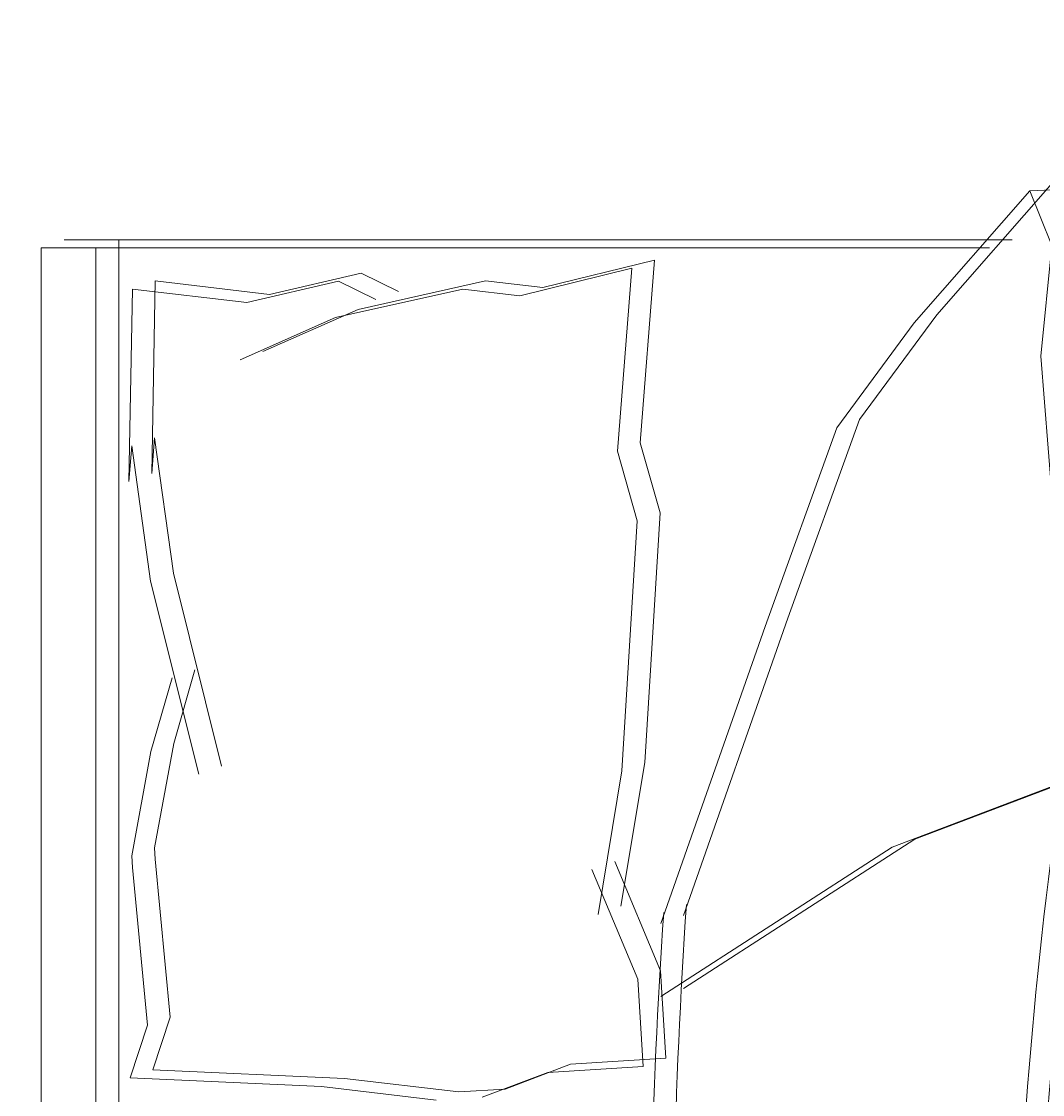
# Model space of a CAD drawing. Units: inches. Extents: x 1962 to 2771, y 1245 to 2660.
# Tile 45 of 114: x 2093 to 2116, y 2098 to 2122. Entities that reach past the tile are written whole.
import ezdxf

# ---------------------------------------------------------------- set-up
doc = ezdxf.new("R2010")
doc.units = ezdxf.units.IN
doc.layers.add('A-ANNO-DIMS', color=2, linetype='Continuous', lineweight=18)
doc.layers.add('A-FURN', color=8, linetype='Continuous', lineweight=13)
doc.styles.get("Standard").update_dxf_attribs({"font": 'arial.ttf'})
doc.dimstyles.get("Standard").update_dxf_attribs({"dimtxt": 0.18, "dimasz": 0.18, "dimexe": 0.18, "dimexo": 0.0625, "dimgap": 0.09, "dimtad": 0, "dimtih": 1, "dimtoh": 1, "dimdec": 4, "dimzin": 0, "dimdsep": 46, "dimtxsty": 'Standard', "dimcen": 0.09, "dimadec": 0, "dimazin": 0, "dimtfac": 1, "dimtdec": 4, "dimtofl": 0, "dimtmove": 0, "dimatfit": 3, "dimfxl": 1, "dimtolj": 1, "dimtzin": 0, "dimarcsym": 0})

# ---------------------------------------------------------------- blocks, each defined once
blk = doc.blocks.new('BED-PLAN')
for p, q in [((22.563, 42.207), (19.979, 39.261)), ((22.563, 42.206), (19.979, 39.261)), ((22.055, 42.025), (19.471, 39.08)), ((22.055, 42.025), (19.471, 39.08)), ((23.442, 42.088), (22.055, 42.025, 3.077)), ((23.442, 42.088), (22.055, 42.025, 3.077)), ((22.547, 40.803), (22.055, 42.025)), ((22.547, 40.803), (22.055, 42.025)), ((0.508, 40.933), (21.66, 40.933)), ((0.508, 40.933), (21.66, 40.933)), ((1.727, 2.945), (1.727, 40.933)), ((1.727, 2.945), (1.727, 40.933)), ((0, 40.752), (21.152, 40.752)), ((0, 40.751), (21.152, 40.751)), ((0, 2.764), (0, 40.751)), ((1.219, 2.764), (1.219, 40.752)), ((1.219, 2.763), (1.219, 40.751)), ((22.301, 38.341), (22.547, 40.803)), ((22.301, 38.341), (22.547, 40.803)), ((13.682, 40.482), (11.187, 39.866)), ((13.682, 40.482), (11.187, 39.866)), ((13.361, 36.403), (13.682, 40.482)), ((13.361, 36.403), (13.682, 40.482)), ((13.173, 40.301), (10.679, 39.684)), ((13.173, 40.301), (10.679, 39.684)), ((12.853, 36.222), (13.173, 40.301)), ((12.853, 36.221), (13.173, 40.301)), ((2.541, 40.016), (2.464, 35.722)), ((2.541, 40.016), (2.464, 35.722)), ((2.541, 40.016), (5.093, 39.715)), ((2.541, 40.016), (5.093, 39.715)), ((4.585, 39.534), (6.628, 40.007)), ((4.585, 39.533), (6.628, 40.007)), ((5.093, 39.715), (7.136, 40.188)), ((5.093, 39.715), (7.136, 40.188)), ((6.628, 40.007), (7.46, 39.598)), ((6.628, 40.007), (7.46, 39.598)), ((9.911, 40.016), (7.072, 39.378)), ((9.911, 40.016), (7.072, 39.378)), ((7.136, 40.188), (7.968, 39.78)), ((7.136, 40.188), (7.968, 39.78)), ((11.187, 39.866), (9.911, 40.016)), ((11.187, 39.866), (9.911, 40.016)), ((2.033, 39.835), (1.955, 35.54)), ((2.033, 39.834), (1.956, 35.54)), ((2.033, 39.835), (4.585, 39.534)), ((2.033, 39.834), (4.585, 39.533)), ((9.402, 39.835), (6.563, 39.197)), ((9.402, 39.835), (6.563, 39.197)), ((10.679, 39.684), (9.402, 39.835)), ((10.679, 39.684), (9.402, 39.835)), ((7.072, 39.378), (4.942, 38.439)), ((7.072, 39.378), (4.942, 38.439)), ((19.979, 39.261), (18.257, 36.922)), ((19.979, 39.261), (18.257, 36.922)), ((6.563, 39.197), (4.434, 38.258)), ((6.563, 39.197), (4.434, 38.258)), ((19.471, 39.08), (17.749, 36.741)), ((19.471, 39.08), (17.749, 36.741)), ((22.547, 35.263), (22.301, 38.341)), ((22.547, 35.263), (22.301, 38.341)), ((18.257, 36.922), (16.658, 32.49)), ((18.257, 36.922), (16.658, 32.49)), ((17.749, 36.741), (16.149, 32.309)), ((17.749, 36.741), (16.149, 32.309)), ((2.464, 35.722), (2.529, 36.519)), ((2.464, 35.722), (2.529, 36.519)), ((2.529, 36.519), (2.948, 33.5)), ((2.529, 36.519), (2.948, 33.5)), ((13.804, 34.845), (13.361, 36.403)), ((13.804, 34.845), (13.361, 36.403)), ((1.955, 35.54), (2.021, 36.338)), ((1.956, 35.54), (2.021, 36.337)), ((2.021, 36.338), (2.44, 33.319)), ((2.021, 36.337), (2.44, 33.318)), ((13.296, 34.663), (12.853, 36.222)), ((13.296, 34.663), (12.853, 36.221)), ((13.461, 29.273), (13.804, 34.845)), ((13.461, 29.273), (13.804, 34.845)), ((12.953, 29.091), (13.296, 34.663)), ((12.953, 29.091), (13.296, 34.663)), ((2.44, 33.319), (3.515, 29.011)), ((2.44, 33.318), (3.515, 29.011)), ((2.948, 33.5), (4.023, 29.192)), ((2.948, 33.5), (4.023, 29.192)), ((16.658, 32.49), (14.326, 25.863)), ((16.658, 32.49), (14.326, 25.862)), ((16.149, 32.309), (13.818, 25.681)), ((16.149, 32.309), (13.818, 25.681)), ((2.92, 31.161), (2.447, 29.52)), ((2.92, 31.161), (2.447, 29.519)), ((3.428, 31.343), (2.955, 29.701)), ((3.428, 31.342), (2.955, 29.701)), ((2.955, 29.701), (2.525, 27.372)), ((2.955, 29.701), (2.525, 27.372)), ((2.447, 29.52), (2.017, 27.19)), ((2.447, 29.519), (2.017, 27.19)), ((12.931, 26.068), (13.461, 29.273)), ((12.931, 26.068), (13.461, 29.273)), ((12.423, 25.886), (12.953, 29.091)), ((12.423, 25.886), (12.953, 29.091)), ((18.979, 27.385), (22.547, 28.739)), ((18.979, 27.384), (22.547, 28.739)), ((19.487, 27.566), (23.055, 28.92)), ((19.487, 27.566), (23.055, 28.92)), ((14.326, 24.236), (19.487, 27.566)), ((14.326, 24.235), (19.487, 27.566)), ((2.525, 27.372), (2.541, 27.117)), ((2.525, 27.372), (2.541, 27.116)), ((13.818, 24.054), (18.979, 27.385)), ((13.818, 24.054), (18.979, 27.384)), ((2.017, 27.19), (2.033, 26.935)), ((2.017, 27.19), (2.033, 26.935)), ((2.541, 27.117), (2.876, 23.597)), ((2.541, 27.116), (2.876, 23.597)), ((13.814, 24.626), (12.793, 27.067)), ((13.814, 24.626), (12.793, 27.066)), ((2.033, 26.935), (2.368, 23.415)), ((2.033, 26.935), (2.368, 23.415)), ((13.306, 24.444), (12.285, 26.885)), ((13.306, 24.444), (12.285, 26.885)), ((13.428, 22.495), (13.306, 24.444)), ((13.428, 22.495), (13.306, 24.444)), ((13.936, 22.676), (13.814, 24.626)), ((13.936, 22.676), (13.814, 24.626)), ((2.876, 23.597), (2.489, 22.421)), ((2.876, 23.597), (2.489, 22.421)), ((2.368, 23.415), (1.981, 22.24)), ((2.368, 23.415), (1.981, 22.24)), ((10.346, 21.991), (11.809, 22.543)), ((10.346, 21.991), (11.809, 22.543)), ((11.809, 22.543), (13.936, 22.676)), ((11.809, 22.543), (13.936, 22.676)), ((2.489, 22.421), (6.762, 22.228)), ((2.489, 22.421), (6.762, 22.228)), ((9.838, 21.81), (11.301, 22.362)), ((9.838, 21.81), (11.301, 22.362)), ((11.301, 22.362), (13.428, 22.495)), ((11.301, 22.362), (13.428, 22.495)), ((1.981, 22.24), (6.254, 22.046)), ((1.981, 22.24), (6.254, 22.046)), ((6.254, 22.046), (8.806, 21.745)), ((6.254, 22.046), (8.806, 21.745)), ((6.762, 22.228), (9.314, 21.927)), ((6.762, 22.228), (9.314, 21.927)), ((9.314, 21.927), (10.346, 21.991)), ((9.314, 21.927), (10.346, 21.991))]:
    blk.add_line(p, q)
for centre, radius, start, end in [((124.254, 14.115), 102.556, 171.78449, 186.90062), ((124.254, 14.115), 102.556, 171.78449, 186.90062), ((124.762, 14.297), 102.556, 171.78449, 186.90062), ((124.762, 14.296), 102.556, 171.78449, 186.90062), ((145.219, 17.161), 131.131, 176.08655, 186.78213), ((145.219, 17.161), 131.131, 176.08655, 186.78213), ((144.711, 16.979), 131.131, 176.08655, 186.78213), ((144.711, 16.979), 131.131, 176.08655, 186.78213)]:
    blk.add_arc(centre, radius, start, end)
blk = doc.blocks.new('*D40')
at = {"layer": 'A-ANNO-DIMS', "color": 0, "lineweight": -2, "transparency": 16777216}
for p, q in [((2072.02, 2033.906), (2072.02, 2583.474)), ((2072.2, 2583.294), (2366.02, 2583.294)), ((2660.627, 2583.294), (2366.808, 2583.294)), ((2660.807, 2524.406), (2660.807, 2583.474))]:
    blk.add_line(p, q, dxfattribs=at)
at = {"layer": 'A-ANNO-DIMS', "color": 0, "transparency": 16777216}
for points in [[(2072.2, 2583.324), (2072.2, 2583.264), (2072.02, 2583.294)], [(2660.627, 2583.324), (2660.627, 2583.264), (2660.807, 2583.294)]]:
    blk.add_solid(points, dxfattribs=at)
at = {"layer": 'Defpoints', "color": 0, "transparency": 16777216}
for p in [(2660.807, 2583.294), (2660.807, 2524.344), (2072.02, 2033.844)]:
    blk.add_point(p, dxfattribs=at)
at = {"layer": 'A-ANNO-DIMS', "color": 0, "transparency": 16777216, "insert": (2366.414, 2583.294), "char_height": 0.18, "attachment_point": 5}
blk.add_mtext('\\A1;588.8', dxfattribs=at)

msp = doc.modelspace()

# ---------------------------------------------------------------- block references
at = {"layer": 'A-FURN'}
msp.add_blockref('BED-PLAN', (2093.917, 2076.454), dxfattribs=at)

# ---------------------------------------------------------------- dimensions: what is measured, and where the dimension line sits
at = {"layer": 'A-ANNO-DIMS'}
dim = msp.add_linear_dim(base=(2660.8074, 2583.2937), p1=(2072.0204, 2033.8437), p2=(2660.8074, 2524.3437), dimstyle='Standard', override={"dimdec": 1, "dimlfac": 1, "dimrnd": 0, "dimzin": 0, "dimdsep": 46, "dimlunit": 2}, dxfattribs=at)
dim.commit()
dim.dimension.update_dxf_attribs({"geometry": '*D40', "text_midpoint": (2366.4139, 2583.2937)})

doc.saveas('drawing.dxf')
